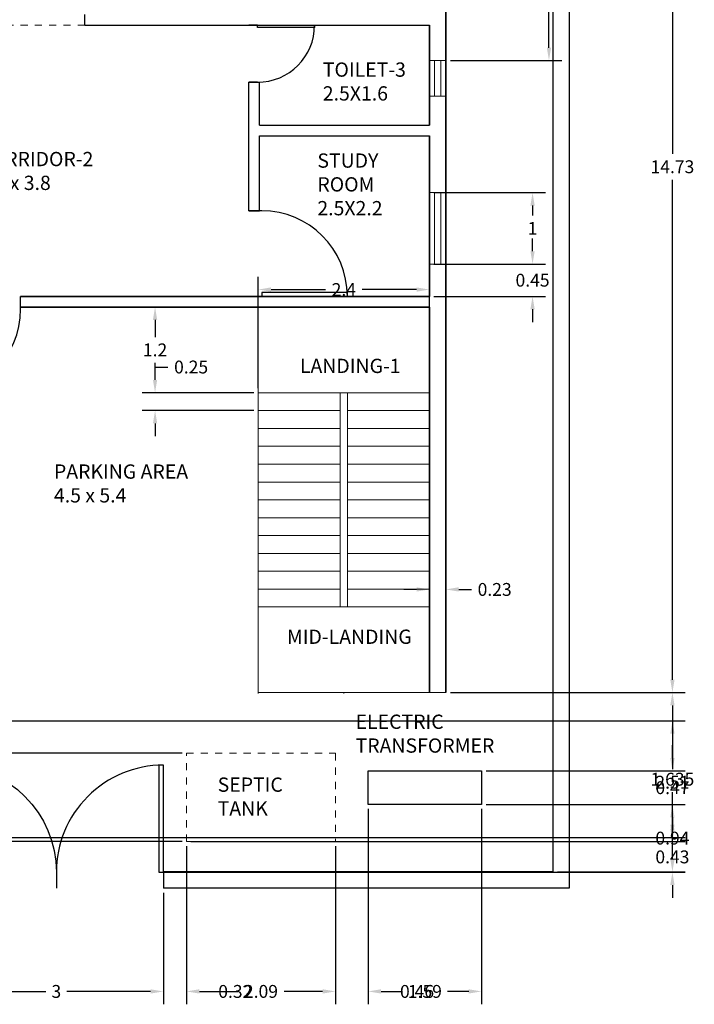
# Model space of a CAD drawing. Units: metres. Extents: x 2527.9 to 2558.5, y 2010.7 to 2033.1.
# Tile 2 of 3: x 2549.1 to 2558.5, y 2010.7 to 2024.5. Entities that reach past the tile are written whole.
import ezdxf

# ---------------------------------------------------------------- set-up
doc = ezdxf.new("R2010")
doc.units = ezdxf.units.M
doc.linetypes.add('ACAD_ISO02W100', pattern=[15, 12, -3])
for name, color, linetype, lineweight in [('A-ANNO-DIMS', 2, 'Continuous', 18), ('A-AREA-IDEN', 180, 'Continuous', 18), ('A-DOOR', 249, 'Continuous', 25), ('A-GLAZ', 249, 'Continuous', 18), ('A-WALL-OVHD', 6, 'ACAD_ISO02W100', 18), ('AC &V', 211, 'Continuous', 18), ('ANNOTATION', 180, 'Continuous', 18), ('C-SITE-GATE', 249, 'Continuous', 25), ('C-SITE-WALL', 110, 'Continuous', 30), ('E-POWR-EQPM', 7, 'Continuous', 25), ('E-POWR-PATT', 7, 'Continuous', 13), ('INNER WALL', 109, 'Continuous', 30), ('OUTER WALL', 110, 'Continuous', 35), ('P-SSWR-TANK', 7, 'ACAD_ISO02W100', 18), ('STAIR CASE', 242, 'Continuous', 18)]:
    doc.layers.add(name, color=color, linetype=linetype, lineweight=lineweight)
doc.styles.get("Standard").update_dxf_attribs({"font": 'arial.ttf'})
doc.dimstyles.get("Standard").update_dxf_attribs({"dimtxt": 0.18, "dimasz": 0.18, "dimexe": 0.18, "dimexo": 0.0625, "dimgap": 0.09, "dimtad": 0, "dimtih": 1, "dimtoh": 1, "dimdec": 1, "dimzin": 0, "dimdsep": 46, "dimtxsty": 'Standard', "dimcen": 0.09, "dimadec": 0, "dimazin": 0, "dimtfac": 1, "dimtdec": 1, "dimtofl": 0, "dimtmove": 0, "dimatfit": 3, "dimfxl": 1, "dimtolj": 1, "dimtzin": 0, "dimarcsym": 0})

# ---------------------------------------------------------------- blocks, each defined once
blk = doc.blocks.new('*U2')
for p, q in [((0, 0), (0, -6)), ((40, 0), (40, -6))]:
    blk.add_line(p, q)
blk.add_lwpolyline([(0, 0), (0, 40), (1.75, 40), (1.75, 0)], close=True)
blk.add_arc((0, 0), 40, 0, 90)
blk = doc.blocks.new('*U5')
for p, q in [((0, 0), (0, -6)), ((-40, 0), (-40, -6))]:
    blk.add_line(p, q)
blk.add_lwpolyline([(0, 0), (0, 40), (-1.75, 40), (-1.75, 0)], close=True)
blk.add_arc((0, 0), 40, 90, 180)
blk = doc.blocks.new('*U6')
for p, q in [((0, 0), (0, 6)), ((40, 0), (40, 6))]:
    blk.add_line(p, q)
blk.add_lwpolyline([(0, 0), (0, -40), (1.75, -40), (1.75, 0)], close=True)
blk.add_arc((0, 0), 40, 270, 0)
blk = doc.blocks.new('VENT-500')
at = {"ltscale": 0.2}
for p, q in [((0, 0), (0, 0.5)), ((0.23, 0.5), (0, 0.5)), ((0.07, 0), (0.07, 0.5)), ((0.16, 0.5), (0.16, 0)), ((0.23, 0.5), (0.23, 0)), ((0.23, 0), (0, 0))]:
    blk.add_line(p, q, dxfattribs=at)
blk = doc.blocks.new('*D20')
at = {"layer": 'A-ANNO-DIMS', "color": 0, "lineweight": -2, "ltscale": 0.2, "transparency": 16777216}
for p, q in [((2555.086, 2029.785), (2558.378, 2029.785)), ((2558.198, 2029.605), (2558.198, 2022.602)), ((2558.198, 2015.235), (2558.198, 2022.238)), ((2555.086, 2015.055), (2558.378, 2015.055))]:
    blk.add_line(p, q, dxfattribs=at)
at = {"layer": 'A-ANNO-DIMS', "color": 0, "lineweight": -3, "ltscale": 0.2, "transparency": 16777216}
for points in [[(2558.168, 2029.605), (2558.228, 2029.605), (2558.198, 2029.785)], [(2558.168, 2015.235), (2558.228, 2015.235), (2558.198, 2015.055)]]:
    blk.add_solid(points, dxfattribs=at)
at = {"layer": 'Defpoints', "color": 0, "lineweight": -3, "ltscale": 0.2, "transparency": 16777216}
for p in [(2555.023, 2029.785), (2558.198, 2029.785), (2555.023, 2015.055)]:
    blk.add_point(p, dxfattribs=at)
at = {"layer": 'A-ANNO-DIMS', "color": 0, "ltscale": 0.2, "transparency": 16777216, "insert": (2558.198, 2022.42), "char_height": 0.18, "attachment_point": 5}
blk.add_mtext('\\A1;14.73', dxfattribs=at)
blk = doc.blocks.new('*D23')
at = {"layer": 'A-ANNO-DIMS', "color": 0, "lineweight": -2, "ltscale": 0.2, "transparency": 16777216}
for p, q in [((2555.086, 2015.055), (2558.378, 2015.055)), ((2558.198, 2014.875), (2558.198, 2013.981)), ((2558.198, 2012.725), (2558.198, 2013.618)), ((2556.586, 2012.545), (2558.378, 2012.545))]:
    blk.add_line(p, q, dxfattribs=at)
at = {"layer": 'A-ANNO-DIMS', "color": 0, "lineweight": -3, "ltscale": 0.2, "transparency": 16777216}
for points in [[(2558.168, 2014.875), (2558.228, 2014.875), (2558.198, 2015.055)], [(2558.168, 2012.725), (2558.228, 2012.725), (2558.198, 2012.545)]]:
    blk.add_solid(points, dxfattribs=at)
at = {"layer": 'Defpoints', "color": 0, "lineweight": -3, "ltscale": 0.2, "transparency": 16777216}
for p in [(2555.023, 2015.055), (2556.523, 2012.545), (2558.198, 2012.545)]:
    blk.add_point(p, dxfattribs=at)
at = {"layer": 'A-ANNO-DIMS', "color": 0, "ltscale": 0.2, "transparency": 16777216, "insert": (2558.198, 2013.8), "char_height": 0.18, "attachment_point": 5}
blk.add_mtext('\\A1;2.51', dxfattribs=at)
blk = doc.blocks.new('*D24')
at = {"layer": 'A-ANNO-DIMS', "color": 0, "lineweight": -2, "ltscale": 0.2, "transparency": 16777216}
for p, q in [((2548.064, 2012.252), (2548.064, 2010.69)), ((2551.064, 2012.252), (2551.064, 2010.69)), ((2548.244, 2010.87), (2549.416, 2010.87)), ((2550.884, 2010.87), (2549.713, 2010.87))]:
    blk.add_line(p, q, dxfattribs=at)
at = {"layer": 'A-ANNO-DIMS', "color": 0, "lineweight": -3, "ltscale": 0.2, "transparency": 16777216}
for points in [[(2548.244, 2010.9), (2548.244, 2010.84), (2548.064, 2010.87)], [(2550.884, 2010.9), (2550.884, 2010.84), (2551.064, 2010.87)]]:
    blk.add_solid(points, dxfattribs=at)
at = {"layer": 'Defpoints', "color": 0, "lineweight": -3, "ltscale": 0.2, "transparency": 16777216}
for p in [(2548.064, 2012.315), (2551.064, 2012.315), (2551.064, 2010.87)]:
    blk.add_point(p, dxfattribs=at)
at = {"layer": 'A-ANNO-DIMS', "color": 0, "ltscale": 0.2, "transparency": 16777216, "insert": (2549.564, 2010.87), "char_height": 0.18, "attachment_point": 5}
blk.add_mtext('\\A1;3', dxfattribs=at)
blk = doc.blocks.new('*D31')
at = {"layer": 'A-ANNO-DIMS', "color": 0, "lineweight": -2, "ltscale": 0.2, "transparency": 16777216}
for p, q in [((2551.389, 2012.905), (2551.389, 2010.69)), ((2551.064, 2012.252), (2551.064, 2010.69)), ((2550.884, 2010.87), (2550.704, 2010.87)), ((2551.569, 2010.87), (2551.749, 2010.87))]:
    blk.add_line(p, q, dxfattribs=at)
at = {"layer": 'A-ANNO-DIMS', "color": 0, "lineweight": -3, "ltscale": 0.2, "transparency": 16777216}
for points in [[(2550.884, 2010.9), (2550.884, 2010.84), (2551.064, 2010.87)], [(2551.569, 2010.9), (2551.569, 2010.84), (2551.389, 2010.87)]]:
    blk.add_solid(points, dxfattribs=at)
at = {"layer": 'Defpoints', "color": 0, "lineweight": -3, "ltscale": 0.2, "transparency": 16777216}
for p in [(2551.389, 2012.968), (2551.064, 2012.315), (2551.389, 2010.87)]:
    blk.add_point(p, dxfattribs=at)
at = {"layer": 'A-ANNO-DIMS', "color": 0, "ltscale": 0.2, "transparency": 16777216, "insert": (2552.072, 2010.87), "char_height": 0.18, "attachment_point": 5}
blk.add_mtext('\\A1;0.32', dxfattribs=at)
blk = doc.blocks.new('*D32')
at = {"layer": 'A-ANNO-DIMS', "color": 0, "lineweight": -2, "ltscale": 0.2, "transparency": 16777216}
for p, q in [((2551.389, 2012.905), (2551.389, 2010.69)), ((2553.475, 2012.905), (2553.475, 2010.69)), ((2551.569, 2010.87), (2552.107, 2010.87)), ((2553.295, 2010.87), (2552.758, 2010.87))]:
    blk.add_line(p, q, dxfattribs=at)
at = {"layer": 'A-ANNO-DIMS', "color": 0, "lineweight": -3, "ltscale": 0.2, "transparency": 16777216}
for points in [[(2551.569, 2010.9), (2551.569, 2010.84), (2551.389, 2010.87)], [(2553.295, 2010.9), (2553.295, 2010.84), (2553.475, 2010.87)]]:
    blk.add_solid(points, dxfattribs=at)
at = {"layer": 'Defpoints', "color": 0, "lineweight": -3, "ltscale": 0.2, "transparency": 16777216}
for p in [(2551.389, 2012.968), (2553.475, 2012.968), (2553.475, 2010.87)]:
    blk.add_point(p, dxfattribs=at)
at = {"layer": 'A-ANNO-DIMS', "color": 0, "ltscale": 0.2, "transparency": 16777216, "insert": (2552.432, 2010.87), "char_height": 0.18, "attachment_point": 5}
blk.add_mtext('\\A1;2.09', dxfattribs=at)
blk = doc.blocks.new('*D33')
at = {"layer": 'A-ANNO-DIMS', "color": 0, "lineweight": -2, "ltscale": 0.2, "transparency": 16777216}
for p, q in [((2553.935, 2013.426), (2553.935, 2010.69)), ((2553.475, 2012.905), (2553.475, 2010.69)), ((2553.295, 2010.87), (2553.115, 2010.87)), ((2554.115, 2010.87), (2554.295, 2010.87))]:
    blk.add_line(p, q, dxfattribs=at)
at = {"layer": 'A-ANNO-DIMS', "color": 0, "lineweight": -3, "ltscale": 0.2, "transparency": 16777216}
for points in [[(2553.295, 2010.9), (2553.295, 2010.84), (2553.475, 2010.87)], [(2554.115, 2010.9), (2554.115, 2010.84), (2553.935, 2010.87)]]:
    blk.add_solid(points, dxfattribs=at)
at = {"layer": 'Defpoints', "color": 0, "lineweight": -3, "ltscale": 0.2, "transparency": 16777216}
for p in [(2553.935, 2013.489), (2553.475, 2012.968), (2553.935, 2010.87)]:
    blk.add_point(p, dxfattribs=at)
at = {"layer": 'A-ANNO-DIMS', "color": 0, "ltscale": 0.2, "transparency": 16777216, "insert": (2554.619, 2010.87), "char_height": 0.18, "attachment_point": 5}
blk.add_mtext('\\A1;0.46', dxfattribs=at)
blk = doc.blocks.new('*D34')
at = {"layer": 'A-ANNO-DIMS', "color": 0, "lineweight": -2, "ltscale": 0.2, "transparency": 16777216}
for p, q in [((2553.935, 2013.426), (2553.935, 2010.69)), ((2555.524, 2013.426), (2555.524, 2010.69)), ((2554.115, 2010.87), (2554.414, 2010.87)), ((2555.344, 2010.87), (2555.045, 2010.87))]:
    blk.add_line(p, q, dxfattribs=at)
at = {"layer": 'A-ANNO-DIMS', "color": 0, "lineweight": -3, "ltscale": 0.2, "transparency": 16777216}
for points in [[(2554.115, 2010.9), (2554.115, 2010.84), (2553.935, 2010.87)], [(2555.344, 2010.9), (2555.344, 2010.84), (2555.524, 2010.87)]]:
    blk.add_solid(points, dxfattribs=at)
at = {"layer": 'Defpoints', "color": 0, "lineweight": -3, "ltscale": 0.2, "transparency": 16777216}
for p in [(2553.935, 2013.489), (2555.524, 2013.489), (2555.524, 2010.87)]:
    blk.add_point(p, dxfattribs=at)
at = {"layer": 'A-ANNO-DIMS', "color": 0, "ltscale": 0.2, "transparency": 16777216, "insert": (2554.729, 2010.87), "char_height": 0.18, "attachment_point": 5}
blk.add_mtext('\\A1;1.59', dxfattribs=at)
blk = doc.blocks.new('*D35')
at = {"layer": 'A-ANNO-DIMS', "color": 0, "lineweight": -2, "ltscale": 0.2, "transparency": 16777216}
for p, q in [((2558.198329, 2014.137896), (2558.198329, 2014.317896)), ((2555.586265, 2013.957896), (2558.378329, 2013.957896)), ((2555.586265, 2013.488734), (2558.378329, 2013.488734)), ((2558.198329, 2013.308734), (2558.198329, 2013.128734))]:
    blk.add_line(p, q, dxfattribs=at)
at = {"layer": 'A-ANNO-DIMS', "color": 0, "lineweight": -3, "ltscale": 0.2, "transparency": 16777216}
for points in [[(2558.168329, 2014.137896), (2558.228329, 2014.137896), (2558.198329, 2013.957896)], [(2558.168329, 2013.308734), (2558.228329, 2013.308734), (2558.198329, 2013.488734)]]:
    blk.add_solid(points, dxfattribs=at)
at = {"layer": 'Defpoints', "color": 0, "lineweight": -3, "ltscale": 0.2, "transparency": 16777216}
for p in [(2555.523765, 2013.957896), (2558.198329, 2013.957896), (2555.523765, 2013.488734)]:
    blk.add_point(p, dxfattribs=at)
at = {"layer": 'A-ANNO-DIMS', "color": 0, "ltscale": 0.2, "transparency": 16777216, "insert": (2558.198329, 2013.723315), "char_height": 0.18, "attachment_point": 5}
blk.add_mtext('\\A1;0.47', dxfattribs=at)
blk = doc.blocks.new('*D37')
at = {"layer": 'A-ANNO-DIMS', "color": 0, "lineweight": -2, "ltscale": 0.2, "transparency": 16777216}
for p, q in [((2545.674, 2014.659), (2558.378, 2014.659)), ((2558.198, 2014.479), (2558.198, 2014.024)), ((2558.198, 2013.204), (2558.198, 2013.66)), ((2545.674, 2013.024), (2558.378, 2013.024))]:
    blk.add_line(p, q, dxfattribs=at)
at = {"layer": 'A-ANNO-DIMS', "color": 0, "lineweight": -3, "ltscale": 0.2, "transparency": 16777216}
for points in [[(2558.168, 2014.479), (2558.228, 2014.479), (2558.198, 2014.659)], [(2558.168, 2013.204), (2558.228, 2013.204), (2558.198, 2013.024)]]:
    blk.add_solid(points, dxfattribs=at)
at = {"layer": 'Defpoints', "color": 0, "lineweight": -3, "ltscale": 0.2, "transparency": 16777216}
for p in [(2545.612, 2014.659), (2558.198, 2014.659), (2545.612, 2013.024)]:
    blk.add_point(p, dxfattribs=at)
at = {"layer": 'A-ANNO-DIMS', "color": 0, "ltscale": 0.2, "transparency": 16777216, "insert": (2558.198, 2013.842), "char_height": 0.18, "attachment_point": 5}
blk.add_mtext('\\A1;1.635', dxfattribs=at)
blk = doc.blocks.new('*D38')
at = {"layer": 'A-ANNO-DIMS', "color": 0, "lineweight": -2, "ltscale": 0.2, "transparency": 16777216}
for p, q in [((2551.326, 2014.205), (2538.928, 2014.205)), ((2539.108, 2014.025), (2539.108, 2013.768)), ((2539.108, 2013.148), (2539.108, 2013.404)), ((2551.326, 2012.968), (2538.928, 2012.968))]:
    blk.add_line(p, q, dxfattribs=at)
at = {"layer": 'A-ANNO-DIMS', "color": 0, "lineweight": -3, "ltscale": 0.2, "transparency": 16777216}
for points in [[(2539.078, 2014.025), (2539.138, 2014.025), (2539.108, 2014.205)], [(2539.078, 2013.148), (2539.138, 2013.148), (2539.108, 2012.968)]]:
    blk.add_solid(points, dxfattribs=at)
at = {"layer": 'Defpoints', "color": 0, "lineweight": -3, "ltscale": 0.2, "transparency": 16777216}
for p in [(2539.108, 2014.205), (2551.389, 2014.205), (2551.389, 2012.968)]:
    blk.add_point(p, dxfattribs=at)
at = {"layer": 'A-ANNO-DIMS', "color": 0, "ltscale": 0.2, "transparency": 16777216, "insert": (2539.108, 2013.586), "char_height": 0.18, "attachment_point": 5}
blk.add_mtext('\\A1;1.237', dxfattribs=at)
blk = doc.blocks.new('*D42')
at = {"layer": 'A-ANNO-DIMS', "color": 0, "lineweight": -2, "ltscale": 0.2, "transparency": 16777216}
for p, q in [((2558.198, 2013.148), (2558.198, 2013.328)), ((2551.451, 2012.968), (2558.378, 2012.968)), ((2551.061, 2012.54), (2558.378, 2012.54)), ((2558.198, 2012.36), (2558.198, 2012.18))]:
    blk.add_line(p, q, dxfattribs=at)
at = {"layer": 'A-ANNO-DIMS', "color": 0, "lineweight": -3, "ltscale": 0.2, "transparency": 16777216}
for points in [[(2558.168, 2013.148), (2558.228, 2013.148), (2558.198, 2012.968)], [(2558.168, 2012.36), (2558.228, 2012.36), (2558.198, 2012.54)]]:
    blk.add_solid(points, dxfattribs=at)
at = {"layer": 'Defpoints', "color": 0, "lineweight": -3, "ltscale": 0.2, "transparency": 16777216}
for p in [(2551.389, 2012.968), (2558.198, 2012.968), (2550.999, 2012.54)]:
    blk.add_point(p, dxfattribs=at)
at = {"layer": 'A-ANNO-DIMS', "color": 0, "ltscale": 0.2, "transparency": 16777216, "insert": (2558.198, 2012.754), "char_height": 0.18, "attachment_point": 5}
blk.add_mtext('\\A1;0.43', dxfattribs=at)
blk = doc.blocks.new('*D43')
at = {"layer": 'A-ANNO-DIMS', "color": 0, "lineweight": -2, "ltscale": 0.2, "transparency": 16777216}
for p, q in [((2555.586, 2013.489), (2558.378, 2013.489)), ((2558.198, 2013.309), (2558.198, 2013.199)), ((2558.198, 2012.725), (2558.198, 2012.835)), ((2556.586, 2012.545), (2558.378, 2012.545))]:
    blk.add_line(p, q, dxfattribs=at)
at = {"layer": 'A-ANNO-DIMS', "color": 0, "lineweight": -3, "ltscale": 0.2, "transparency": 16777216}
for points in [[(2558.168, 2013.309), (2558.228, 2013.309), (2558.198, 2013.489)], [(2558.168, 2012.725), (2558.228, 2012.725), (2558.198, 2012.545)]]:
    blk.add_solid(points, dxfattribs=at)
at = {"layer": 'Defpoints', "color": 0, "lineweight": -3, "ltscale": 0.2, "transparency": 16777216}
for p in [(2555.524, 2013.489), (2556.523, 2012.545), (2558.198, 2012.545)]:
    blk.add_point(p, dxfattribs=at)
at = {"layer": 'A-ANNO-DIMS', "color": 0, "ltscale": 0.2, "transparency": 16777216, "insert": (2558.198, 2013.017), "char_height": 0.18, "attachment_point": 5}
blk.add_mtext('\\A1;0.94', dxfattribs=at)
blk = doc.blocks.new('*D44')
at = {"layer": 'A-ANNO-DIMS', "color": 0, "lineweight": -2, "ltscale": 0.2, "transparency": 16777216}
for p, q in [((2552.393, 2019.317), (2552.393, 2020.88)), ((2554.793, 2019.317), (2554.793, 2020.88)), ((2552.573, 2020.7), (2553.338, 2020.7)), ((2554.613, 2020.7), (2553.848, 2020.7))]:
    blk.add_line(p, q, dxfattribs=at)
at = {"layer": 'A-ANNO-DIMS', "color": 0, "lineweight": -3, "ltscale": 0.2, "transparency": 16777216}
for points in [[(2552.573, 2020.73), (2552.573, 2020.67), (2552.393, 2020.7)], [(2554.613, 2020.73), (2554.613, 2020.67), (2554.793, 2020.7)]]:
    blk.add_solid(points, dxfattribs=at)
at = {"layer": 'Defpoints', "color": 0, "lineweight": -3, "ltscale": 0.2, "transparency": 16777216}
for p in [(2554.793, 2020.7), (2552.393, 2019.255), (2554.793, 2019.255)]:
    blk.add_point(p, dxfattribs=at)
at = {"layer": 'A-ANNO-DIMS', "color": 0, "ltscale": 0.2, "transparency": 16777216, "insert": (2553.593, 2020.7), "char_height": 0.18, "attachment_point": 5}
blk.add_mtext('\\A1;2.4', dxfattribs=at)
blk = doc.blocks.new('*D45')
at = {"layer": 'A-ANNO-DIMS', "color": 0, "lineweight": -2, "ltscale": 0.2, "transparency": 16777216}
for p, q in [((2552.331, 2020.455), (2550.768, 2020.455)), ((2550.948, 2020.275), (2550.948, 2020.035)), ((2550.948, 2019.435), (2550.948, 2019.674)), ((2552.331, 2019.255), (2550.768, 2019.255))]:
    blk.add_line(p, q, dxfattribs=at)
at = {"layer": 'A-ANNO-DIMS', "color": 0, "lineweight": -3, "ltscale": 0.2, "transparency": 16777216}
for points in [[(2550.918, 2020.275), (2550.978, 2020.275), (2550.948, 2020.455)], [(2550.918, 2019.435), (2550.978, 2019.435), (2550.948, 2019.255)]]:
    blk.add_solid(points, dxfattribs=at)
at = {"layer": 'Defpoints', "color": 0, "lineweight": -3, "ltscale": 0.2, "transparency": 16777216}
for p in [(2550.948, 2020.455), (2552.393, 2020.455), (2552.393, 2019.255)]:
    blk.add_point(p, dxfattribs=at)
at = {"layer": 'A-ANNO-DIMS', "color": 0, "ltscale": 0.2, "transparency": 16777216, "insert": (2550.948, 2019.855), "char_height": 0.18, "attachment_point": 5}
blk.add_mtext('\\A1;1.2', dxfattribs=at)
blk = doc.blocks.new('*D46')
at = {"layer": 'A-ANNO-DIMS', "color": 0, "lineweight": -2, "ltscale": 0.2, "transparency": 16777216}
for p, q in [((2550.948, 2019.435), (2550.948, 2019.615)), ((2550.948, 2019.615), (2551.128, 2019.615)), ((2552.331, 2019.255), (2550.768, 2019.255)), ((2552.331, 2019.005), (2550.768, 2019.005)), ((2550.948, 2018.825), (2550.948, 2018.645))]:
    blk.add_line(p, q, dxfattribs=at)
at = {"layer": 'A-ANNO-DIMS', "color": 0, "lineweight": -3, "ltscale": 0.2, "transparency": 16777216}
for points in [[(2550.918, 2019.435), (2550.978, 2019.435), (2550.948, 2019.255)], [(2550.918, 2018.825), (2550.978, 2018.825), (2550.948, 2019.005)]]:
    blk.add_solid(points, dxfattribs=at)
at = {"layer": 'Defpoints', "color": 0, "lineweight": -3, "ltscale": 0.2, "transparency": 16777216}
for p in [(2550.948, 2019.255), (2552.393, 2019.255), (2552.393, 2019.005)]:
    blk.add_point(p, dxfattribs=at)
at = {"layer": 'A-ANNO-DIMS', "color": 0, "ltscale": 0.2, "transparency": 16777216, "insert": (2551.453, 2019.615), "char_height": 0.18, "attachment_point": 5}
blk.add_mtext('\\A1;0.25', dxfattribs=at)
blk = doc.blocks.new('*D48')
at = {"layer": 'A-ANNO-DIMS', "color": 0, "lineweight": -2, "ltscale": 0.2, "transparency": 16777216}
for p, q in [((2554.793, 2015.117), (2554.793, 2016.68)), ((2555.023, 2015.117), (2555.023, 2016.68)), ((2554.613, 2016.5), (2554.433, 2016.5)), ((2555.203, 2016.5), (2555.383, 2016.5))]:
    blk.add_line(p, q, dxfattribs=at)
at = {"layer": 'A-ANNO-DIMS', "color": 0, "lineweight": -3, "ltscale": 0.2, "transparency": 16777216}
for points in [[(2554.613, 2016.53), (2554.613, 2016.47), (2554.793, 2016.5)], [(2555.203, 2016.53), (2555.203, 2016.47), (2555.023, 2016.5)]]:
    blk.add_solid(points, dxfattribs=at)
at = {"layer": 'Defpoints', "color": 0, "lineweight": -3, "ltscale": 0.2, "transparency": 16777216}
for p in [(2555.023, 2016.5), (2554.793, 2015.055), (2555.023, 2015.055)]:
    blk.add_point(p, dxfattribs=at)
at = {"layer": 'A-ANNO-DIMS', "color": 0, "ltscale": 0.2, "transparency": 16777216, "insert": (2555.707, 2016.5), "char_height": 0.18, "attachment_point": 5}
blk.add_mtext('\\A1;0.23', dxfattribs=at)
blk = doc.blocks.new('*D54')
at = {"layer": 'A-ANNO-DIMS', "color": 0, "lineweight": -2, "ltscale": 0.2, "transparency": 16777216}
for p, q in [((2555.086, 2026.316), (2556.648, 2026.316)), ((2556.468, 2026.136), (2556.468, 2025.293)), ((2556.468, 2024.087), (2556.468, 2024.929)), ((2555.086, 2023.907), (2556.648, 2023.907))]:
    blk.add_line(p, q, dxfattribs=at)
at = {"layer": 'A-ANNO-DIMS', "color": 0, "lineweight": -3, "ltscale": 0.2, "transparency": 16777216}
for points in [[(2556.438, 2026.136), (2556.498, 2026.136), (2556.468, 2026.316)], [(2556.438, 2024.087), (2556.498, 2024.087), (2556.468, 2023.907)]]:
    blk.add_solid(points, dxfattribs=at)
at = {"layer": 'Defpoints', "color": 0, "lineweight": -3, "ltscale": 0.2, "transparency": 16777216}
for p in [(2555.023, 2026.316), (2555.023, 2023.907), (2556.468, 2023.907)]:
    blk.add_point(p, dxfattribs=at)
at = {"layer": 'A-ANNO-DIMS', "color": 0, "ltscale": 0.2, "transparency": 16777216, "insert": (2556.468, 2025.111), "char_height": 0.18, "attachment_point": 5}
blk.add_mtext('\\A1;2.409', dxfattribs=at)
blk = doc.blocks.new('*D55')
at = {"layer": 'A-ANNO-DIMS', "color": 0, "lineweight": -2, "ltscale": 0.2, "transparency": 16777216}
for p, q in [((2556.238, 2021.237), (2556.238, 2021.417)), ((2554.856, 2021.057), (2556.418, 2021.057)), ((2554.856, 2020.605), (2556.418, 2020.605)), ((2556.238, 2020.425), (2556.238, 2020.245))]:
    blk.add_line(p, q, dxfattribs=at)
at = {"layer": 'A-ANNO-DIMS', "color": 0, "lineweight": -3, "ltscale": 0.2, "transparency": 16777216}
for points in [[(2556.208, 2021.237), (2556.268, 2021.237), (2556.238, 2021.057)], [(2556.208, 2020.425), (2556.268, 2020.425), (2556.238, 2020.605)]]:
    blk.add_solid(points, dxfattribs=at)
at = {"layer": 'Defpoints', "color": 0, "lineweight": -3, "ltscale": 0.2, "transparency": 16777216}
for p in [(2554.793, 2021.057), (2554.793, 2020.605), (2556.238, 2020.605)]:
    blk.add_point(p, dxfattribs=at)
at = {"layer": 'A-ANNO-DIMS', "color": 0, "ltscale": 0.2, "transparency": 16777216, "insert": (2556.238, 2020.831), "char_height": 0.18, "attachment_point": 5}
blk.add_mtext('\\A1;0.45', dxfattribs=at)
blk = doc.blocks.new('*D56')
at = {"layer": 'A-ANNO-DIMS', "color": 0, "lineweight": -2, "ltscale": 0.2, "transparency": 16777216}
for p, q in [((2554.856, 2022.057), (2556.418, 2022.057)), ((2556.238, 2021.877), (2556.238, 2021.738)), ((2556.238, 2021.237), (2556.238, 2021.377)), ((2554.856, 2021.057), (2556.418, 2021.057))]:
    blk.add_line(p, q, dxfattribs=at)
at = {"layer": 'A-ANNO-DIMS', "color": 0, "lineweight": -3, "ltscale": 0.2, "transparency": 16777216}
for points in [[(2556.208, 2021.877), (2556.268, 2021.877), (2556.238, 2022.057)], [(2556.208, 2021.237), (2556.268, 2021.237), (2556.238, 2021.057)]]:
    blk.add_solid(points, dxfattribs=at)
at = {"layer": 'Defpoints', "color": 0, "lineweight": -3, "ltscale": 0.2, "transparency": 16777216}
for p in [(2554.793, 2022.057), (2554.793, 2021.057), (2556.238, 2021.057)]:
    blk.add_point(p, dxfattribs=at)
at = {"layer": 'A-ANNO-DIMS', "color": 0, "ltscale": 0.2, "transparency": 16777216, "insert": (2556.238, 2021.557), "char_height": 0.18, "attachment_point": 5}
blk.add_mtext('\\A1;1', dxfattribs=at)

msp = doc.modelspace()

# ---------------------------------------------------------------- hatches: boundary and pattern name
at = {"layer": 'E-POWR-PATT', "ltscale": 0.005}
h = msp.add_hatch(dxfattribs=at)
h.set_pattern_fill('ACAD_ISO15W100', color=256)
h.paths.add_polyline_path([(2541.2861, 2014.1352), (2541.2861, 2013.3533), (2543.1643, 2013.3533), (2543.1643, 2014.1352)])
h.paths.add_polyline_path([(2555.5238, 2013.9579), (2553.935, 2013.9579), (2553.935, 2013.4887), (2555.5238, 2013.4887)])

# ---------------------------------------------------------------- linework, layer by layer
at = {"layer": 'A-GLAZ', "ltscale": 0.2}
for p, q in [((2554.7933, 2021.0572), (2554.7933, 2022.0572)), ((2554.7933, 2022.0572), (2555.0233, 2022.0572)), ((2554.8633, 2021.0572), (2554.8633, 2022.0572)), ((2554.9533, 2022.0572), (2554.9533, 2021.0572)), ((2555.0233, 2022.0572), (2555.0233, 2021.0572)), ((2555.0233, 2021.0572), (2554.7933, 2021.0572))]:
    msp.add_line(p, q, dxfattribs=at)
at = {"layer": 'A-WALL-OVHD', "ltscale": 0.002}
msp.add_line((2547.4633, 2024.4045), (2549.9633, 2024.4045), dxfattribs=at)
at = {"layer": 'C-SITE-WALL', "ltscale": 0.5}
msp.add_line((2551.0644, 2012.5445), (2551.0644, 2012.3145), dxfattribs=at)
at = {"layer": 'C-SITE-WALL'}
for points in [[(2556.7533, 2031.5145), (2556.7533, 2012.3145), (2551.0644, 2012.3145)], [(2556.5233, 2031.2845), (2556.5233, 2012.5445), (2551.0644, 2012.5445)]]:
    msp.add_lwpolyline(points, dxfattribs=at)
at = {"layer": 'E-POWR-EQPM', "ltscale": 0.005}
msp.add_lwpolyline([(2553.935, 2013.9579), (2555.5238, 2013.9579), (2555.5238, 2013.4887), (2553.935, 2013.4887)], close=True, dxfattribs=at)
at = {"layer": 'INNER WALL'}
for p, q in [((2549.9633, 2024.4045), (2549.9633, 2024.5545)), ((2549.9633, 2024.4045), (2552.2633, 2024.4045)), ((2552.2633, 2024.4045), (2552.4133, 2024.4045)), ((2552.4133, 2024.4045), (2554.7933, 2024.4045)), ((2552.2633, 2021.8045), (2552.2633, 2023.6045)), ((2552.2633, 2023.6045), (2552.4133, 2023.6045)), ((2552.4133, 2023.0045), (2552.4133, 2023.6045)), ((2552.4133, 2023.0045), (2554.7933, 2023.0045)), ((2552.4133, 2021.8045), (2552.4133, 2022.8545)), ((2552.4133, 2022.8545), (2554.7933, 2022.8545)), ((2552.2633, 2021.8045), (2552.4133, 2021.8045)), ((2549.0633, 2020.4545), (2549.0633, 2020.6045)), ((2552.2633, 2020.6045), (2552.4133, 2020.6045))]:
    msp.add_line(p, q, dxfattribs=at)
at = {"layer": 'OUTER WALL'}
for p, q in [((2555.0233, 2029.7845), (2555.0233, 2015.0545)), ((2554.7933, 2024.4045), (2554.7933, 2023.0045)), ((2554.7933, 2022.8545), (2554.7933, 2020.6045)), ((2549.0633, 2020.6045), (2552.2633, 2020.6045)), ((2552.4133, 2020.6045), (2554.7933, 2020.6045)), ((2549.0633, 2020.4545), (2554.7933, 2020.4545)), ((2554.7933, 2020.4545), (2554.7933, 2015.0545))]:
    msp.add_line(p, q, dxfattribs=at)
at = {"layer": 'P-SSWR-TANK', "ltscale": 0.005}
msp.add_lwpolyline([(2551.3887, 2014.2049), (2553.4754, 2014.2049), (2553.4754, 2012.9678), (2551.3887, 2012.9678)], close=True, dxfattribs=at)
at = {"layer": 'STAIR CASE'}
for p, q in [((2552.3933, 2020.4545), (2552.3933, 2015.0445)), ((2552.3933, 2019.2545), (2554.7933, 2019.2545)), ((2553.5433, 2019.2545), (2553.5433, 2016.2545)), ((2553.6433, 2019.2545), (2553.6433, 2016.2545)), ((2552.3933, 2019.0045), (2553.5433, 2019.0045)), ((2553.6433, 2019.0045), (2554.7933, 2019.0045)), ((2552.3933, 2018.7545), (2553.5433, 2018.7545)), ((2553.6433, 2018.7545), (2554.7933, 2018.7545)), ((2552.3933, 2018.5045), (2553.5433, 2018.5045)), ((2553.6433, 2018.5045), (2554.7933, 2018.5045)), ((2552.3933, 2018.2545), (2553.5433, 2018.2545)), ((2553.6433, 2018.2545), (2554.7933, 2018.2545)), ((2552.3933, 2018.0045), (2553.5433, 2018.0045)), ((2553.6433, 2018.0045), (2554.7933, 2018.0045)), ((2552.3933, 2017.7545), (2553.5433, 2017.7545)), ((2553.6433, 2017.7545), (2554.7933, 2017.7545)), ((2552.3933, 2017.5045), (2553.5433, 2017.5045)), ((2553.6433, 2017.5045), (2554.7933, 2017.5045)), ((2552.3933, 2017.2545), (2553.5433, 2017.2545)), ((2553.6433, 2017.2545), (2554.7933, 2017.2545)), ((2552.3933, 2017.0045), (2553.5433, 2017.0045)), ((2553.6433, 2017.0045), (2554.7933, 2017.0045)), ((2552.3933, 2016.7545), (2553.5433, 2016.7545)), ((2553.6433, 2016.7545), (2554.7933, 2016.7545)), ((2552.3933, 2016.5045), (2553.5433, 2016.5045)), ((2553.6433, 2016.5045), (2554.7933, 2016.5045)), ((2552.3933, 2016.2545), (2554.7933, 2016.2545)), ((2552.3933, 2015.0545), (2555.0233, 2015.0545)), ((2553.5933, 2015.0545), (2553.5933, 2015.0445))]:
    msp.add_line(p, q, dxfattribs=at)

# ---------------------------------------------------------------- block references
at = {"layer": 'A-DOOR'}
for name, p, xscale, yscale, zscale, rotation in [('*U2', (2552.3833, 2024.4045), 0.0199999999999985, 0.0199999999999985, 0.0199999999999985, 270), ('*U5', (2552.4433, 2020.6045), 0.0299999999999995, 0.0299999999999995, 0.0299999999999995, 269.9999999999578), ('*U5', (2547.8633, 2020.4245), 0.0299999999999995, 0.0299999999999995, 0.0299999999999995, 179.9999999999577)]:
    msp.add_blockref(name, p, dxfattribs=dict(at, xscale=xscale, yscale=yscale, zscale=zscale, rotation=rotation))
at = {"layer": 'AC &V'}
msp.add_blockref('VENT-500', (2554.7933, 2023.4067), dxfattribs=at)
at = {"layer": 'C-SITE-GATE', "yscale": 0.0374999999999908, "zscale": 0.0374999999999908}
for p, xscale, rotation in [((2548.0644, 2012.5395), -0.0374999999999908, 180), ((2551.0644, 2012.5395), 0.0374999999999908, 179.9999999999577)]:
    msp.add_blockref('*U6', p, dxfattribs=dict(at, xscale=xscale, rotation=rotation))

# ---------------------------------------------------------------- texts
at = {"layer": 'A-AREA-IDEN', "char_height": 0.2, "attachment_point": 1}
for s, width, heights, insert in [('TOILET-3 2.5X1.6', 1.31727, [0], (2553.2985, 2023.8806)), ('CORRIDOR-2   6.6 x 3.8', 1.770765, [0], (2548.4709, 2022.6278)), ('STUDY ROOM 2.5X2.2', 1.075451, [0], (2553.2224, 2022.6066)), ('LANDING-1', 1.522595, [0], (2552.9776, 2019.731)), ('PARKING AREA\\P4.5 x 5.4', 2.144683, [0.541], (2549.5308, 2018.2511)), ('MID-LANDING', 1.522595, [0], (2552.7963, 2015.9375))]:
    msp.add_mtext_dynamic_manual_height_columns(s, width=width, gutter_width=12.5, heights=heights, dxfattribs=dict(at, insert=insert))
at = {"layer": 'ANNOTATION', "char_height": 0.2, "attachment_point": 1}
for s, width, gutter_width, heights, insert in [('ELECTRIC\\PTRANSFORMER\\P', 2.063815, 0.2422, [0.8274], (2553.7577, 2014.7469)), ('SEPTIC TANK', 1.205045, 12.5, [0.541], (2551.8249, 2013.8661))]:
    msp.add_mtext_dynamic_manual_height_columns(s, width=width, gutter_width=gutter_width, heights=heights, dxfattribs=dict(at, insert=insert))

# ---------------------------------------------------------------- dimensions: what is measured, and where the dimension line sits
at = {"layer": 'A-ANNO-DIMS', "ltscale": 0.2}
for base, p1, p2, angle, override, picture, middle in [((2558.1983, 2029.7845), (2555.0233, 2015.0545), (2555.0233, 2029.7845), 90, {"dimdec": 2, "dimlfac": 1, "dimrnd": 0, "dimzin": 0, "dimdsep": 46, "dimlunit": 2}, '*D20', (2558.1983, 2022.4195)), ((2556.4683, 2023.9067), (2555.0233, 2026.3157), (2555.0233, 2023.9067), 270, {"dimdec": 3, "dimlfac": 1, "dimrnd": 0, "dimzin": 0, "dimdsep": 46, "dimlunit": 2}, '*D54', (2556.4683, 2025.1112)), ((2556.2383, 2021.0572), (2554.7933, 2022.0572), (2554.7933, 2021.0572), 270, {"dimdec": 0, "dimlfac": 1, "dimrnd": 0, "dimzin": 0, "dimdsep": 46, "dimlunit": 2}, '*D56', (2556.2383, 2021.5572)), ((2556.2383, 2020.6045), (2554.7933, 2021.0572), (2554.7933, 2020.6045), 270, {"dimdec": 2, "dimlfac": 1, "dimrnd": 0, "dimzin": 0, "dimdsep": 46, "dimlunit": 2}, '*D55', (2556.2383, 2020.8309)), ((2550.9483, 2020.4545), (2552.3933, 2019.2545), (2552.3933, 2020.4545), 90, {"dimdec": 1, "dimlfac": 1, "dimrnd": 0, "dimzin": 0, "dimdsep": 46, "dimlunit": 2}, '*D45', (2550.9483, 2019.8545)), ((2550.9483, 2019.2545), (2552.3933, 2019.0045), (2552.3933, 2019.2545), 90, {"dimdec": 2, "dimlfac": 1, "dimrnd": 0, "dimzin": 0, "dimdsep": 46, "dimlunit": 2}, '*D46', (2551.4528, 2019.6145)), ((2558.1983, 2012.5445), (2555.0233, 2015.0545), (2556.5233, 2012.5445), 90, {"dimdec": 2, "dimlfac": 1, "dimrnd": 0, "dimzin": 0, "dimdsep": 46, "dimlunit": 2}, '*D23', (2558.1983, 2013.7995)), ((2558.1983, 2014.6594), (2545.6118, 2013.0243), (2545.6118, 2014.6594), 90, {"dimdec": 3, "dimlfac": 1, "dimrnd": 0, "dimzin": 0, "dimdsep": 46, "dimlunit": 2}, '*D37', (2558.1983, 2013.8419)), ((2558.1983, 2013.9579), (2555.5238, 2013.4887), (2555.5238, 2013.9579), 90, {"dimdec": 2, "dimlfac": 1, "dimrnd": 0, "dimzin": 0, "dimdsep": 46, "dimlunit": 2}, '*D35', (2558.1983, 2013.7233)), ((2539.1083, 2014.2049), (2551.3887, 2012.9678), (2551.3887, 2014.2049), 90, {"dimdec": 3, "dimlfac": 1, "dimrnd": 0, "dimzin": 0, "dimdsep": 46, "dimlunit": 2}, '*D38', (2539.1083, 2013.5863)), ((2558.1983, 2012.5445), (2555.5238, 2013.4887), (2556.5233, 2012.5445), 90, {"dimdec": 2, "dimlfac": 1, "dimrnd": 0, "dimzin": 0, "dimdsep": 46, "dimlunit": 2}, '*D43', (2558.1983, 2013.0166)), ((2558.1983, 2012.9678), (2550.9988, 2012.5395), (2551.3887, 2012.9678), 90, {"dimdec": 2, "dimlfac": 1, "dimrnd": 0, "dimzin": 0, "dimdsep": 46, "dimlunit": 2}, '*D42', (2558.1983, 2012.7536))]:
    dim = msp.add_linear_dim(base=base, p1=p1, p2=p2, angle=angle, dimstyle='Standard', override=override, dxfattribs=at)
    dim.commit()
    dim.dimension.update_dxf_attribs({"geometry": picture, "text_midpoint": middle})
for base, p1, p2, override, picture, middle in [((2554.7933, 2020.6995), (2552.3933, 2019.2545), (2554.7933, 2019.2545), {"dimdec": 1, "dimlfac": 1, "dimrnd": 0, "dimzin": 0, "dimdsep": 46, "dimlunit": 2}, '*D44', (2553.5933, 2020.6995)), ((2555.0233, 2016.4995), (2554.7933, 2015.0545), (2555.0233, 2015.0545), {"dimdec": 2, "dimlfac": 1, "dimrnd": 0, "dimzin": 0, "dimdsep": 46, "dimlunit": 2}, '*D48', (2555.7071, 2016.4995)), ((2553.935, 2010.8695), (2553.4754, 2012.9678), (2553.935, 2013.4887), {"dimdec": 2, "dimlfac": 1, "dimrnd": 0, "dimzin": 0, "dimdsep": 46, "dimlunit": 2}, '*D33', (2554.6187, 2010.8695)), ((2555.5238, 2010.8695), (2553.935, 2013.4887), (2555.5238, 2013.4887), {"dimdec": 2, "dimlfac": 1, "dimrnd": 0, "dimzin": 0, "dimdsep": 46, "dimlunit": 2}, '*D34', (2554.7294, 2010.8695)), ((2551.3887, 2010.8695), (2551.0644, 2012.3145), (2551.3887, 2012.9678), {"dimdec": 2, "dimlfac": 1, "dimrnd": 0, "dimzin": 0, "dimdsep": 46, "dimlunit": 2}, '*D31', (2552.0716, 2010.8695)), ((2553.4754, 2010.8695), (2551.3887, 2012.9678), (2553.4754, 2012.9678), {"dimdec": 2, "dimlfac": 1, "dimrnd": 0, "dimzin": 0, "dimdsep": 46, "dimlunit": 2}, '*D32', (2552.432, 2010.8695)), ((2551.0644, 2010.8695), (2548.0644, 2012.3145), (2551.0644, 2012.3145), {"dimdec": 0, "dimlfac": 1, "dimrnd": 0, "dimzin": 0, "dimdsep": 46, "dimlunit": 2}, '*D24', (2549.5644, 2010.8695))]:
    dim = msp.add_linear_dim(base=base, p1=p1, p2=p2, dimstyle='Standard', override=override, dxfattribs=at)
    dim.commit()
    dim.dimension.update_dxf_attribs({"geometry": picture, "text_midpoint": middle})

doc.saveas('drawing.dxf')
